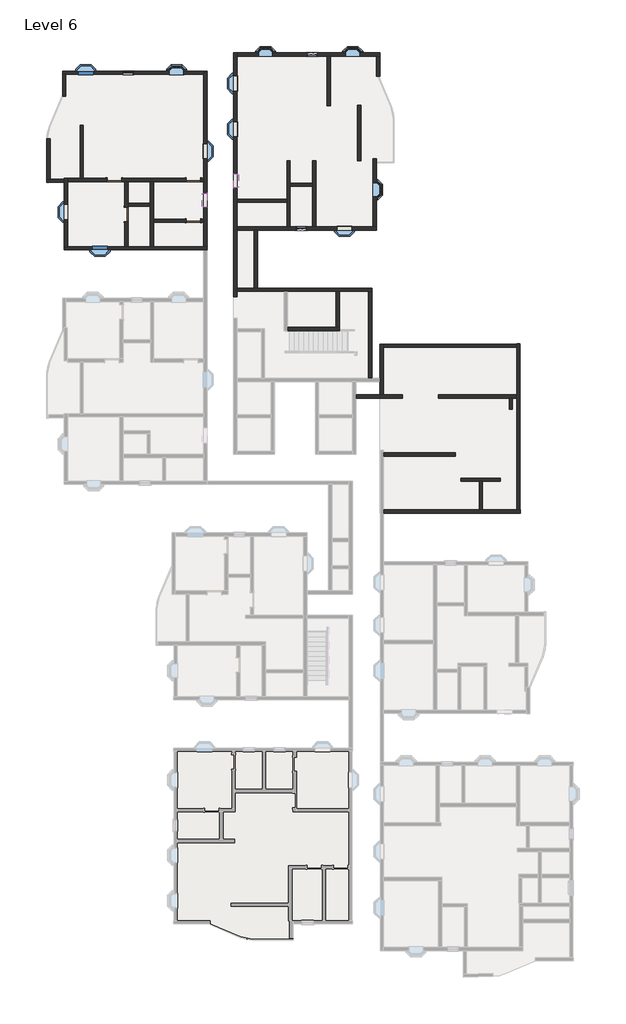
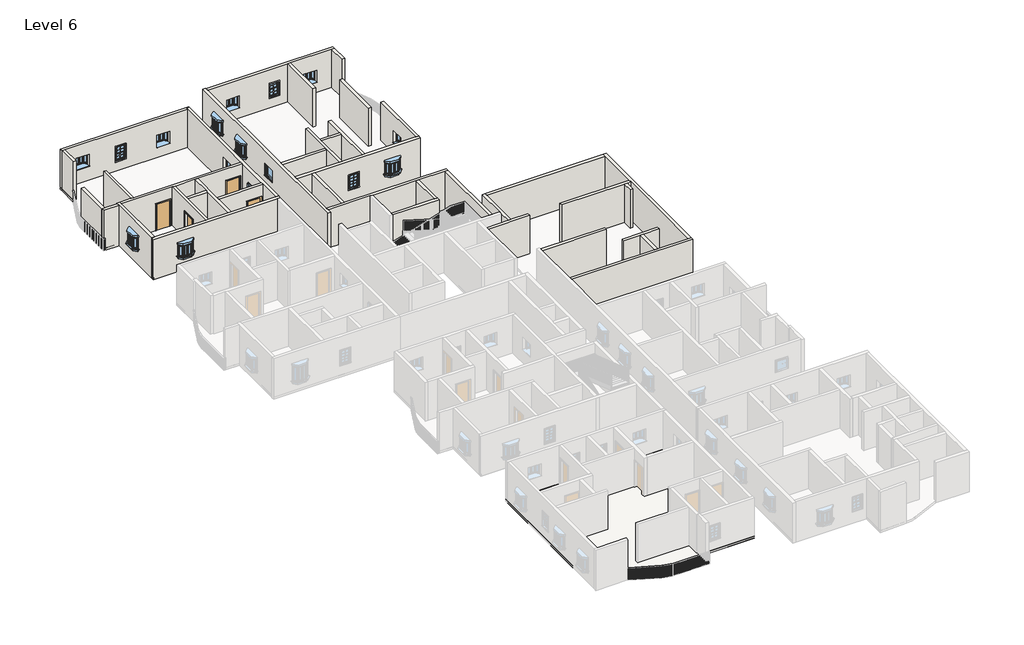
# One storey, part 4 of 14: 39 walls, 16 windows, 4 doors, 2 roofs.
# Revit data of these elements (continued)
# Element 32 (IfcWall, "9\" w") (continued)
#   Top Offset = 0' - 0"
#   Base Offset = 0' - 0"
#   wall height = 10' - 0"
#   Phase Created = New Construction
#   Base Constraint = Level 6
#   Top Constraint = Level 7
#   Materials on its faces: "Default Wall", "Grass"
# Element 33 (IfcWall, "9\" w")
#   Top Offset = 0' - 0"
#   Base Offset = 0' - 0"
#   wall height = 10' - 0"
#   Phase Created = New Construction
#   Base Constraint = Level 6
#   Top Constraint = Level 7
#   Materials on its faces: "Default Wall", "Brick, Soldier Course", "Earth"
# Element 34 (IfcWall, "9\" w")
#   Top Offset = 0' - 0"
#   Base Offset = 0' - 0"
#   wall height = 10' - 0"
#   Phase Created = New Construction
#   Base Constraint = Level 6
#   Top Constraint = Level 7
#   Materials on its faces: "Default Wall", "Earth"
# Element 35 (IfcWall, "9\" w")
#   Top Offset = 0' - 0"
#   Base Offset = 0' - 0"
#   wall height = 10' - 0"
#   Phase Created = New Construction
#   Base Constraint = Level 6
#   Top Constraint = Level 7
#   Materials on its faces: "Default Wall", "Parking Stripe"
# Elements 36, 37, 38 (IfcWall, "9\" w")
#   Top Offset = 0' - 0"
#   Base Offset = 0' - 0"
#   wall height = 10' - 0"
#   Phase Created = New Construction
#   Base Constraint = Level 6
#   Top Constraint = Level 7
#   Materials on its faces: "Default Wall", "Window Frame"
# Element 43 (IfcWall, "9\" w")
#   Top Offset = 0' - 0"
#   Base Offset = 0' - 0"
#   wall height = 10' - 0"
#   Phase Created = New Construction
#   Base Constraint = Level 6
#   Top Constraint = Level 7
#   Materials on its faces: "Default Wall", "Parking Stripe", "Default Mass Interior Wall"
# Element 44 (IfcWall, "9\" w")
#   Top Offset = 0' - 0"
#   Base Offset = 0' - 0"
#   wall height = 10' - 0"
#   Phase Created = New Construction
#   Base Constraint = Level 6
#   Top Constraint = Level 7
#   Materials on its faces: "Default Wall", "Parking Stripe", "Brick, Soldier Course"
# Element 46 (IfcWindow, "910x910mm")
#   Mark = "307"
#   Phase Created = New Construction
#   Materials on its faces: "Window Frame", "Glass"
# Element 47 (IfcWindow, "910x910mm")
#   Mark = "308"
#   Phase Created = New Construction
#   Materials on its faces: "Window Frame", "Glass"
# Element 48 (IfcWindow, "910x910mm")
#   Mark = "309"
#   Phase Created = New Construction
#   Materials on its faces: "Window Frame", "Glass"
# Element 49 (IfcWindow, "910x910mm")
#   Mark = "339"
#   Phase Created = New Construction
#   Materials on its faces: "Window Frame", "Glass"
# Element 50 (IfcWindow, "910x910mm")
#   Mark = "340"
#   Phase Created = New Construction
#   Materials on its faces: "Window Frame", "Glass"
# Element 51 (IfcWindow, "910x910mm")
#   Mark = "472"
#   Phase Created = New Construction
#   Materials on its faces: "Window Frame", "Glass"
# Element 52 (IfcWindow, "910x910mm")
#   Mark = "473"
#   Phase Created = New Construction
#   Materials on its faces: "Window Frame", "Glass"
# Element 53 (IfcWindow, "910x910mm")
#   Mark = "481"
#   Phase Created = New Construction
#   Materials on its faces: "Window Frame", "Glass"
# Element 54 (IfcWindow, "910x910mm")
#   Mark = "482"
#   Phase Created = New Construction
#   Materials on its faces: "Window Frame", "Glass"
# Element 55 (IfcWindow, "910x910mm")
#   Mark = "341"
#   Phase Created = New Construction
#   Materials on its faces: "Window Frame", "Glass"
# Element 56 (IfcWindow, "910x910mm")
#   Mark = "342"
#   Phase Created = New Construction
#   Materials on its faces: "Window Frame", "Glass"
# Element 57 (IfcWindow, "Window-Double-Hung : 26\" x 42\"")
#   Mark = "474"
#   Window Inset = 0' - 0"
#   Interior Wall Closure = 0' - 1 1/2"
#   Frame Extension = 0' - 1 1/4"
#   Exterior Wall Closure = 0' - 0 1/2"
#   Interior Trim Visibility = yes
#   Indicator Visibility = yes
#   Exterior Trim Visibility = yes
#   Phase Created = New Construction
#   Materials on its faces: "Wood - Stained", "Glass", "Clad - White"
# Element 58 (IfcWindow, "Window-Double-Hung : 26\" x 42\"")
#   Mark = "483"
#   Window Inset = 0' - 0"
#   Interior Wall Closure = 0' - 1 1/2"
#   Frame Extension = 0' - 1 1/4"
#   Exterior Wall Closure = 0' - 0 1/2"
#   Interior Trim Visibility = yes
#   Indicator Visibility = yes
#   Exterior Trim Visibility = yes
#   Phase Created = New Construction
#   Materials on its faces: "Wood - Stained", "Glass", "Clad - White"
# Element 59 (IfcWindow, "Window-Double-Hung : 26\" x 42\"")
#   Mark = "360"
#   Window Inset = 0' - 0"
#   Interior Wall Closure = 0' - 1 1/2"
#   Frame Extension = 0' - 1 1/4"
#   Exterior Wall Closure = 0' - 0 1/2"
#   Interior Trim Visibility = yes
#   Indicator Visibility = yes
#   Exterior Trim Visibility = yes
#   Phase Created = New Construction
#   Materials on its faces: "Wood - Stained", "Glass", "Clad - White"
# Element 60 (IfcWindow, "Windows_Sgl_w-Glazing_Bars : 910x910mm")
#   Mark = "343"
#   Phase Created = New Construction
#   Materials on its faces: "Window Frame", "Glass"
# Element 61 (IfcWindow, "Windows_Sgl_w-Glazing_Bars : 910x910mm")
#   Mark = "347"
#   Phase Created = New Construction
#   Materials on its faces: "Window Frame", "Glass"
# Materials
#   "Door - Panel": class "Wood", colour RGB 210 159 95, transparency 0, Cost = 0
#   "Door - Frame": colour RGB 118 70 51, transparency 0, Cost = 0
#   "Window Frame": colour RGB 249 249 249, transparency 0
#   "Glass": class "Glass", colour RGB 0 128 192, transparency 0.75, Description = "Soda Lime Glass", Cost = 0
#   "Wood - Stained": class "Wood", colour RGB 224 178 126, transparency 0, Cost = 0
#   "Clad - White": class "Wood", colour RGB 242 242 238, transparency 0, Cost = 0
#   "Default Roof": colour RGB 88 101 114, transparency 0, Cost = 0
#   "Default Wall": colour RGB 128 128 128, transparency 0, Cost = 0
#   "Grass": class "Generic", colour RGB 104 137 66, transparency 0, Description = "Physical material.", Cost = 0
#   "Parking Stripe": class "Paint", colour RGB 250 250 91, transparency 0, Cost = 0
#   "Carpet (1)": class "Carpet", colour RGB 124 80 67, transparency 0, Description = "Interior finish", Cost = 0
#   "Brick, Soldier Course": class "Masonry", colour RGB 170 98 104, transparency 0, Description = "Common brick soldier coursed", Cost = 0
#   "Default Mass Interior Wall": class "Generic", colour RGB 195 229 126, transparency 0, Cost = 0
#   "Earth": class "Generic", colour RGB 97 75 62, transparency 0, Description = "Soil", Cost = 0
